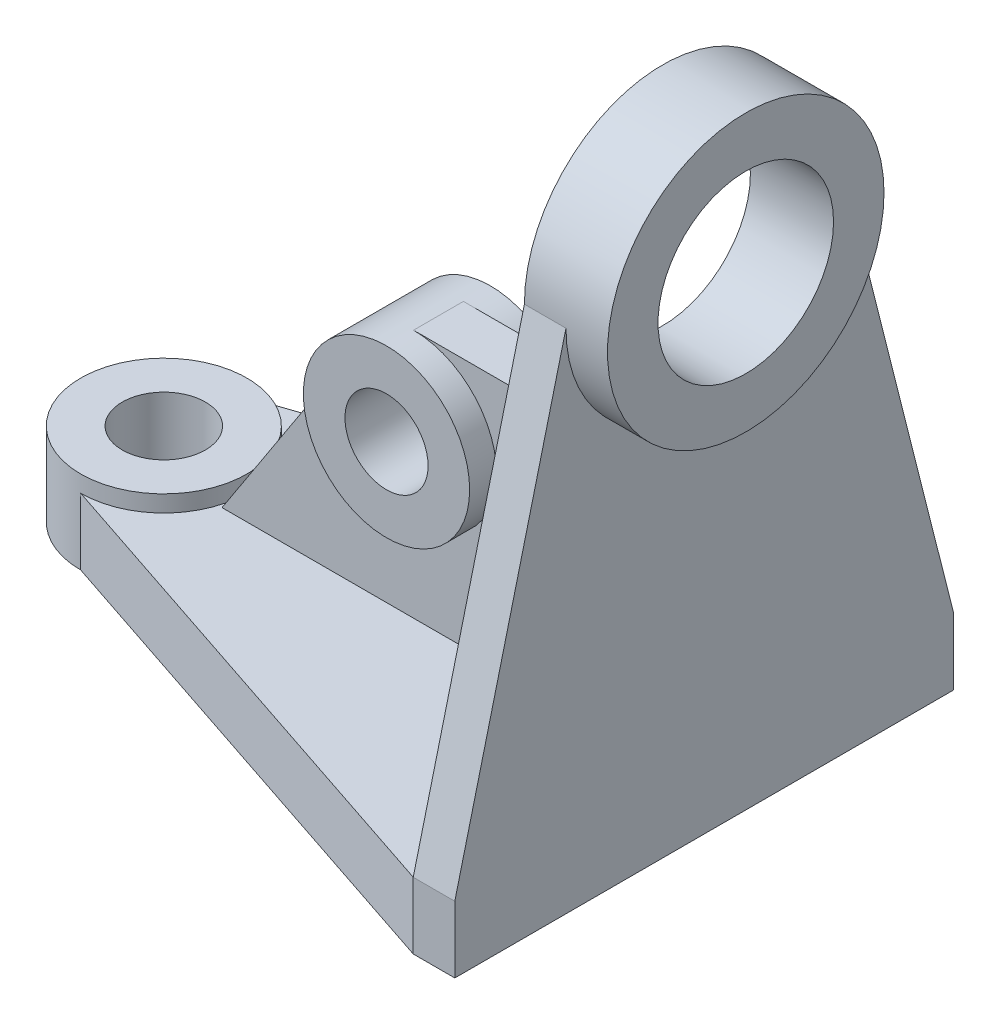
ISO-10303-21;
HEADER;
FILE_DESCRIPTION(('STEP AP214'),'2;1');
FILE_NAME('part.step','',(''),(''),'','','');
FILE_SCHEMA(('AUTOMOTIVE_DESIGN { 1 0 10303 214 1 1 1 1 }'));
ENDSEC;
DATA;
#1=APPLICATION_CONTEXT('core data for automotive mechanical design processes');
#2=APPLICATION_PROTOCOL_DEFINITION('international standard','automotive_design',2000,#1);
#3=PRODUCT_CONTEXT('',#1,'mechanical');
#4=PRODUCT('Part','Part','',(#3));
#5=PRODUCT_RELATED_PRODUCT_CATEGORY('part','',(#4));
#6=PRODUCT_DEFINITION_FORMATION('','',#4);
#7=PRODUCT_DEFINITION_CONTEXT('part definition',#1,'design');
#8=PRODUCT_DEFINITION('design','',#6,#7);
#9=PRODUCT_DEFINITION_SHAPE('','',#8);
#10=(LENGTH_UNIT() NAMED_UNIT(*) SI_UNIT(.MILLI.,.METRE.));
#11=(NAMED_UNIT(*) PLANE_ANGLE_UNIT() SI_UNIT($,.RADIAN.));
#12=(NAMED_UNIT(*) SI_UNIT($,.STERADIAN.) SOLID_ANGLE_UNIT());
#13=UNCERTAINTY_MEASURE_WITH_UNIT(LENGTH_MEASURE(1.E-05),#10,'distance_accuracy_value','');
#14=(GEOMETRIC_REPRESENTATION_CONTEXT(3) GLOBAL_UNCERTAINTY_ASSIGNED_CONTEXT((#13)) GLOBAL_UNIT_ASSIGNED_CONTEXT((#10,
#11,#12)) REPRESENTATION_CONTEXT('',''));
#15=CARTESIAN_POINT('',(0.,0.,0.));
#16=DIRECTION('',(0.,0.,1.));
#17=DIRECTION('',(1.,0.,0.));
#18=AXIS2_PLACEMENT_3D('',#15,#16,#17);
#19=CARTESIAN_POINT('',(0.,16.,0.));
#20=DIRECTION('',(0.,-1.,0.));
#21=DIRECTION('',(0.,0.,-1.));
#22=AXIS2_PLACEMENT_3D('',#19,#20,#21);
#23=PLANE('',#22);
#24=DIRECTION('',(1.,0.,0.));
#25=VECTOR('',#24,1.);
#26=CARTESIAN_POINT('',(120.,16.,6.));
#27=LINE('',#26,#25);
#28=CARTESIAN_POINT('',(20.,16.,6.));
#29=VERTEX_POINT('',#28);
#30=CARTESIAN_POINT('',(120.,16.,6.));
#31=VERTEX_POINT('',#30);
#32=EDGE_CURVE('E287',#29,#31,#27,.T.);
#33=ORIENTED_EDGE('',*,*,#32,.F.);
#34=DIRECTION('',(0.,0.,-1.));
#35=VECTOR('',#34,1.);
#36=CARTESIAN_POINT('',(20.,16.,6.));
#37=LINE('',#36,#35);
#38=CARTESIAN_POINT('',(20.,16.,0.));
#39=VERTEX_POINT('',#38);
#40=EDGE_CURVE('E170',#29,#39,#37,.T.);
#41=ORIENTED_EDGE('',*,*,#40,.T.);
#42=CARTESIAN_POINT('',(0.,16.,0.));
#43=DIRECTION('',(0.,-1.,0.));
#44=DIRECTION('',(0.,0.,-1.));
#45=AXIS2_PLACEMENT_3D('',#42,#43,#44);
#46=CIRCLE('',#45,20.);
#47=CARTESIAN_POINT('',(0.,16.,20.));
#48=VERTEX_POINT('',#47);
#49=EDGE_CURVE('E64',#39,#48,#46,.T.);
#50=ORIENTED_EDGE('',*,*,#49,.T.);
#51=DIRECTION('',(0.948683298050514,0.,0.316227766016838));
#52=VECTOR('',#51,1.);
#53=CARTESIAN_POINT('',(0.,16.,20.));
#54=LINE('',#53,#52);
#55=CARTESIAN_POINT('',(120.,16.,60.));
#56=VERTEX_POINT('',#55);
#57=EDGE_CURVE('E217',#48,#56,#54,.T.);
#58=ORIENTED_EDGE('',*,*,#57,.T.);
#59=DIRECTION('',(0.,0.,-1.));
#60=VECTOR('',#59,1.);
#61=CARTESIAN_POINT('',(120.,16.,0.));
#62=LINE('',#61,#60);
#63=EDGE_CURVE('E189',#56,#31,#62,.T.);
#64=ORIENTED_EDGE('',*,*,#63,.T.);
#65=EDGE_LOOP('',(#33,#41,#50,#58,#64));
#66=FACE_BOUND('',#65,.T.);
#67=ADVANCED_FACE('F41',(#66),#23,.F.);
#68=CARTESIAN_POINT('',(20.,16.,-6.));
#69=VERTEX_POINT('',#68);
#70=EDGE_CURVE('E163',#39,#69,#37,.T.);
#71=ORIENTED_EDGE('',*,*,#70,.T.);
#72=DIRECTION('',(1.,0.,0.));
#73=VECTOR('',#72,1.);
#74=CARTESIAN_POINT('',(120.,16.,-6.));
#75=LINE('',#74,#73);
#76=CARTESIAN_POINT('',(120.,16.,-6.));
#77=VERTEX_POINT('',#76);
#78=EDGE_CURVE('E294',#69,#77,#75,.T.);
#79=ORIENTED_EDGE('',*,*,#78,.T.);
#80=CARTESIAN_POINT('',(120.,16.,-60.));
#81=VERTEX_POINT('',#80);
#82=EDGE_CURVE('E187',#77,#81,#62,.T.);
#83=ORIENTED_EDGE('',*,*,#82,.T.);
#84=DIRECTION('',(-0.948683298050514,0.,0.316227766016838));
#85=VECTOR('',#84,1.);
#86=CARTESIAN_POINT('',(0.,16.,-20.));
#87=LINE('',#86,#85);
#88=CARTESIAN_POINT('',(0.,16.,-20.));
#89=VERTEX_POINT('',#88);
#90=EDGE_CURVE('E209',#81,#89,#87,.T.);
#91=ORIENTED_EDGE('',*,*,#90,.T.);
#92=EDGE_CURVE('E214',#89,#39,#46,.T.);
#93=ORIENTED_EDGE('',*,*,#92,.T.);
#94=EDGE_LOOP('',(#71,#79,#83,#91,#93));
#95=FACE_BOUND('',#94,.T.);
#96=ADVANCED_FACE('F301',(#95),#23,.F.);
#97=CARTESIAN_POINT('',(120.,0.,0.));
#98=DIRECTION('',(1.,0.,0.));
#99=DIRECTION('',(0.,0.,-1.));
#100=AXIS2_PLACEMENT_3D('',#97,#98,#99);
#101=PLANE('',#100);
#102=CARTESIAN_POINT('',(120.,122.,0.));
#103=DIRECTION('',(1.,0.,0.));
#104=DIRECTION('',(0.,0.,-1.));
#105=AXIS2_PLACEMENT_3D('',#102,#103,#104);
#106=CIRCLE('',#105,21.1123106954547);
#107=CARTESIAN_POINT('',(120.,122.,-21.1123106954547));
#108=VERTEX_POINT('',#107);
#109=EDGE_CURVE('E171',#108,#108,#106,.T.);
#110=ORIENTED_EDGE('',*,*,#109,.T.);
#111=EDGE_LOOP('',(#110));
#112=FACE_BOUND('',#111,.T.);
#113=DIRECTION('',(0.,1.,0.));
#114=VECTOR('',#113,1.);
#115=CARTESIAN_POINT('',(120.,76.,6.));
#116=LINE('',#115,#114);
#117=CARTESIAN_POINT('',(120.,76.,6.));
#118=VERTEX_POINT('',#117);
#119=EDGE_CURVE('E161',#31,#118,#116,.T.);
#120=ORIENTED_EDGE('',*,*,#119,.F.);
#121=ORIENTED_EDGE('',*,*,#63,.F.);
#122=DIRECTION('',(0.,0.969620280754232,-0.244615026419239));
#123=VECTOR('',#122,1.);
#124=CARTESIAN_POINT('',(120.,15.1884056140009,60.2047483804881));
#125=LINE('',#124,#123);
#126=CARTESIAN_POINT('',(120.,122.,33.2584050528832));
#127=VERTEX_POINT('',#126);
#128=EDGE_CURVE('E182',#56,#127,#125,.T.);
#129=ORIENTED_EDGE('',*,*,#128,.T.);
#130=CARTESIAN_POINT('',(120.,122.,0.));
#131=DIRECTION('',(1.,0.,0.));
#132=DIRECTION('',(0.,0.,-1.));
#133=AXIS2_PLACEMENT_3D('',#130,#131,#132);
#134=CIRCLE('',#133,33.2584050528832);
#135=CARTESIAN_POINT('',(120.,122.,-33.2584050528833));
#136=VERTEX_POINT('',#135);
#137=EDGE_CURVE('E174',#136,#127,#134,.T.);
#138=ORIENTED_EDGE('',*,*,#137,.F.);
#139=DIRECTION('',(0.,0.969620280754232,0.244615026419239));
#140=VECTOR('',#139,1.);
#141=CARTESIAN_POINT('',(120.,15.1884056140009,-60.2047483804881));
#142=LINE('',#141,#140);
#143=EDGE_CURVE('E192',#81,#136,#142,.T.);
#144=ORIENTED_EDGE('',*,*,#143,.F.);
#145=ORIENTED_EDGE('',*,*,#82,.F.);
#146=DIRECTION('',(0.,1.,0.));
#147=VECTOR('',#146,1.);
#148=CARTESIAN_POINT('',(120.,76.,-6.));
#149=LINE('',#148,#147);
#150=CARTESIAN_POINT('',(120.,76.,-6.));
#151=VERTEX_POINT('',#150);
#152=EDGE_CURVE('E154',#77,#151,#149,.T.);
#153=ORIENTED_EDGE('',*,*,#152,.T.);
#154=DIRECTION('',(0.,0.,-1.));
#155=VECTOR('',#154,1.);
#156=CARTESIAN_POINT('',(120.,76.,6.));
#157=LINE('',#156,#155);
#158=EDGE_CURVE('E148',#118,#151,#157,.T.);
#159=ORIENTED_EDGE('',*,*,#158,.F.);
#160=EDGE_LOOP('',(#120,#121,#129,#138,#144,#145,#153,#159));
#161=FACE_BOUND('',#160,.T.);
#162=ADVANCED_FACE('F281',(#112,#161),#101,.F.);
#163=CARTESIAN_POINT('',(0.,20.,0.));
#164=DIRECTION('',(0.,-1.,0.));
#165=DIRECTION('',(0.,0.,-1.));
#166=AXIS2_PLACEMENT_3D('',#163,#164,#165);
#167=CYLINDRICAL_SURFACE('',#166,20.);
#168=CARTESIAN_POINT('',(0.,20.,0.));
#169=DIRECTION('',(0.,1.,0.));
#170=DIRECTION('',(0.,0.,1.));
#171=AXIS2_PLACEMENT_3D('',#168,#169,#170);
#172=CIRCLE('',#171,20.);
#173=CARTESIAN_POINT('',(0.,20.,20.));
#174=VERTEX_POINT('',#173);
#175=EDGE_CURVE('E47',#174,#174,#172,.T.);
#176=ORIENTED_EDGE('',*,*,#175,.F.);
#177=EDGE_LOOP('',(#176));
#178=FACE_BOUND('',#177,.T.);
#179=DIRECTION('',(0.,-1.,0.));
#180=VECTOR('',#179,1.);
#181=CARTESIAN_POINT('',(0.,16.,-20.));
#182=LINE('',#181,#180);
#183=CARTESIAN_POINT('',(0.,0.,-20.));
#184=VERTEX_POINT('',#183);
#185=EDGE_CURVE('E239',#89,#184,#182,.T.);
#186=ORIENTED_EDGE('',*,*,#185,.T.);
#187=CARTESIAN_POINT('',(0.,0.,0.));
#188=DIRECTION('',(0.,1.,0.));
#189=DIRECTION('',(0.,0.,1.));
#190=AXIS2_PLACEMENT_3D('',#187,#188,#189);
#191=CIRCLE('',#190,20.);
#192=CARTESIAN_POINT('',(0.,0.,20.));
#193=VERTEX_POINT('',#192);
#194=EDGE_CURVE('E254',#184,#193,#191,.T.);
#195=ORIENTED_EDGE('',*,*,#194,.T.);
#196=DIRECTION('',(0.,-1.,0.));
#197=VECTOR('',#196,1.);
#198=CARTESIAN_POINT('',(0.,16.,20.));
#199=LINE('',#198,#197);
#200=EDGE_CURVE('E240',#48,#193,#199,.T.);
#201=ORIENTED_EDGE('',*,*,#200,.F.);
#202=ORIENTED_EDGE('',*,*,#49,.F.);
#203=ORIENTED_EDGE('',*,*,#92,.F.);
#204=EDGE_LOOP('',(#186,#195,#201,#202,#203));
#205=FACE_BOUND('',#204,.T.);
#206=ADVANCED_FACE('F43',(#178,#205),#167,.T.);
#207=CARTESIAN_POINT('',(0.,20.,0.));
#208=DIRECTION('',(0.,1.,0.));
#209=DIRECTION('',(0.,0.,1.));
#210=AXIS2_PLACEMENT_3D('',#207,#208,#209);
#211=PLANE('',#210);
#212=ORIENTED_EDGE('',*,*,#175,.T.);
#213=EDGE_LOOP('',(#212));
#214=FACE_BOUND('',#213,.T.);
#215=CARTESIAN_POINT('',(0.,20.,0.));
#216=DIRECTION('',(0.,1.,0.));
#217=DIRECTION('',(0.,0.,1.));
#218=AXIS2_PLACEMENT_3D('',#215,#216,#217);
#219=CIRCLE('',#218,10.);
#220=CARTESIAN_POINT('',(0.,20.,10.));
#221=VERTEX_POINT('',#220);
#222=EDGE_CURVE('E249',#221,#221,#219,.T.);
#223=ORIENTED_EDGE('',*,*,#222,.F.);
#224=EDGE_LOOP('',(#223));
#225=FACE_BOUND('',#224,.T.);
#226=ADVANCED_FACE('F361',(#214,#225),#211,.T.);
#227=CARTESIAN_POINT('',(0.,0.,0.));
#228=DIRECTION('',(0.,1.,0.));
#229=DIRECTION('',(0.,0.,1.));
#230=AXIS2_PLACEMENT_3D('',#227,#228,#229);
#231=PLANE('',#230);
#232=ORIENTED_EDGE('',*,*,#194,.F.);
#233=DIRECTION('',(-0.948683298050514,0.,0.316227766016838));
#234=VECTOR('',#233,1.);
#235=CARTESIAN_POINT('',(0.,0.,-20.));
#236=LINE('',#235,#234);
#237=CARTESIAN_POINT('',(120.,0.,-60.));
#238=VERTEX_POINT('',#237);
#239=EDGE_CURVE('E228',#238,#184,#236,.T.);
#240=ORIENTED_EDGE('',*,*,#239,.F.);
#241=DIRECTION('',(-1.,0.,0.));
#242=VECTOR('',#241,1.);
#243=CARTESIAN_POINT('',(120.,0.,-60.));
#244=LINE('',#243,#242);
#245=CARTESIAN_POINT('',(130.,0.,-60.));
#246=VERTEX_POINT('',#245);
#247=EDGE_CURVE('E221',#246,#238,#244,.T.);
#248=ORIENTED_EDGE('',*,*,#247,.F.);
#249=DIRECTION('',(0.,0.,-1.));
#250=VECTOR('',#249,1.);
#251=CARTESIAN_POINT('',(130.,0.,-60.));
#252=LINE('',#251,#250);
#253=CARTESIAN_POINT('',(130.,0.,60.));
#254=VERTEX_POINT('',#253);
#255=EDGE_CURVE('E201',#254,#246,#252,.T.);
#256=ORIENTED_EDGE('',*,*,#255,.F.);
#257=DIRECTION('',(1.,0.,0.));
#258=VECTOR('',#257,1.);
#259=CARTESIAN_POINT('',(130.,0.,60.));
#260=LINE('',#259,#258);
#261=CARTESIAN_POINT('',(120.,0.,60.));
#262=VERTEX_POINT('',#261);
#263=EDGE_CURVE('E208',#262,#254,#260,.T.);
#264=ORIENTED_EDGE('',*,*,#263,.F.);
#265=DIRECTION('',(0.948683298050514,0.,0.316227766016838));
#266=VECTOR('',#265,1.);
#267=CARTESIAN_POINT('',(0.,0.,20.));
#268=LINE('',#267,#266);
#269=EDGE_CURVE('E230',#193,#262,#268,.T.);
#270=ORIENTED_EDGE('',*,*,#269,.F.);
#271=EDGE_LOOP('',(#232,#240,#248,#256,#264,#270));
#272=FACE_BOUND('',#271,.T.);
#273=CARTESIAN_POINT('',(0.,0.,0.));
#274=DIRECTION('',(0.,1.,0.));
#275=DIRECTION('',(0.,0.,1.));
#276=AXIS2_PLACEMENT_3D('',#273,#274,#275);
#277=CIRCLE('',#276,10.);
#278=CARTESIAN_POINT('',(0.,0.,10.));
#279=VERTEX_POINT('',#278);
#280=EDGE_CURVE('E248',#279,#279,#277,.T.);
#281=ORIENTED_EDGE('',*,*,#280,.T.);
#282=EDGE_LOOP('',(#281));
#283=FACE_BOUND('',#282,.T.);
#284=ADVANCED_FACE('F269',(#272,#283),#231,.F.);
#285=CARTESIAN_POINT('',(0.,20.,0.));
#286=DIRECTION('',(0.,-1.,0.));
#287=DIRECTION('',(0.,0.,-1.));
#288=AXIS2_PLACEMENT_3D('',#285,#286,#287);
#289=CYLINDRICAL_SURFACE('',#288,10.);
#290=ORIENTED_EDGE('',*,*,#222,.T.);
#291=EDGE_LOOP('',(#290));
#292=FACE_BOUND('',#291,.T.);
#293=ORIENTED_EDGE('',*,*,#280,.F.);
#294=EDGE_LOOP('',(#293));
#295=FACE_BOUND('',#294,.T.);
#296=ADVANCED_FACE('F360',(#292,#295),#289,.F.);
#297=CARTESIAN_POINT('',(130.,16.,-60.));
#298=DIRECTION('',(-1.,0.,0.));
#299=DIRECTION('',(0.,0.,1.));
#300=AXIS2_PLACEMENT_3D('',#297,#298,#299);
#301=PLANE('',#300);
#302=ORIENTED_EDGE('',*,*,#255,.T.);
#303=DIRECTION('',(0.,-1.,0.));
#304=VECTOR('',#303,1.);
#305=CARTESIAN_POINT('',(130.,16.,-60.));
#306=LINE('',#305,#304);
#307=CARTESIAN_POINT('',(130.,16.,-60.));
#308=VERTEX_POINT('',#307);
#309=EDGE_CURVE('E246',#308,#246,#306,.T.);
#310=ORIENTED_EDGE('',*,*,#309,.F.);
#311=DIRECTION('',(0.,0.969620280754232,0.244615026419239));
#312=VECTOR('',#311,1.);
#313=CARTESIAN_POINT('',(130.,15.1884056140009,-60.2047483804881));
#314=LINE('',#313,#312);
#315=CARTESIAN_POINT('',(130.,122.,-33.2584050528832));
#316=VERTEX_POINT('',#315);
#317=EDGE_CURVE('E190',#308,#316,#314,.T.);
#318=ORIENTED_EDGE('',*,*,#317,.T.);
#319=CARTESIAN_POINT('',(130.,122.,0.));
#320=DIRECTION('',(1.,0.,0.));
#321=DIRECTION('',(0.,0.,-1.));
#322=AXIS2_PLACEMENT_3D('',#319,#320,#321);
#323=CIRCLE('',#322,33.2584050528832);
#324=CARTESIAN_POINT('',(130.,122.,33.2584050528832));
#325=VERTEX_POINT('',#324);
#326=EDGE_CURVE('E181',#325,#316,#323,.T.);
#327=ORIENTED_EDGE('',*,*,#326,.F.);
#328=DIRECTION('',(0.,0.969620280754232,-0.244615026419239));
#329=VECTOR('',#328,1.);
#330=CARTESIAN_POINT('',(130.,15.1884056140009,60.2047483804881));
#331=LINE('',#330,#329);
#332=CARTESIAN_POINT('',(130.,16.,60.));
#333=VERTEX_POINT('',#332);
#334=EDGE_CURVE('E197',#333,#325,#331,.T.);
#335=ORIENTED_EDGE('',*,*,#334,.F.);
#336=DIRECTION('',(0.,-1.,0.));
#337=VECTOR('',#336,1.);
#338=CARTESIAN_POINT('',(130.,16.,60.));
#339=LINE('',#338,#337);
#340=EDGE_CURVE('E222',#333,#254,#339,.T.);
#341=ORIENTED_EDGE('',*,*,#340,.T.);
#342=EDGE_LOOP('',(#302,#310,#318,#327,#335,#341));
#343=FACE_BOUND('',#342,.T.);
#344=ADVANCED_FACE('F273',(#343),#301,.F.);
#345=CARTESIAN_POINT('',(120.,16.,-60.));
#346=DIRECTION('',(0.,0.,1.));
#347=DIRECTION('',(1.,0.,0.));
#348=AXIS2_PLACEMENT_3D('',#345,#346,#347);
#349=PLANE('',#348);
#350=ORIENTED_EDGE('',*,*,#247,.T.);
#351=DIRECTION('',(0.,-1.,0.));
#352=VECTOR('',#351,1.);
#353=CARTESIAN_POINT('',(120.,16.,-60.));
#354=LINE('',#353,#352);
#355=EDGE_CURVE('E243',#81,#238,#354,.T.);
#356=ORIENTED_EDGE('',*,*,#355,.F.);
#357=DIRECTION('',(-1.,0.,0.));
#358=VECTOR('',#357,1.);
#359=CARTESIAN_POINT('',(120.,16.,-60.));
#360=LINE('',#359,#358);
#361=EDGE_CURVE('E207',#308,#81,#360,.T.);
#362=ORIENTED_EDGE('',*,*,#361,.F.);
#363=ORIENTED_EDGE('',*,*,#309,.T.);
#364=EDGE_LOOP('',(#350,#356,#362,#363));
#365=FACE_BOUND('',#364,.T.);
#366=ADVANCED_FACE('F354',(#365),#349,.F.);
#367=CARTESIAN_POINT('',(0.,16.,-20.));
#368=DIRECTION('',(0.316227766016838,0.,0.948683298050514));
#369=DIRECTION('',(0.948683298050514,0.,-0.316227766016838));
#370=AXIS2_PLACEMENT_3D('',#367,#368,#369);
#371=PLANE('',#370);
#372=ORIENTED_EDGE('',*,*,#239,.T.);
#373=ORIENTED_EDGE('',*,*,#185,.F.);
#374=ORIENTED_EDGE('',*,*,#90,.F.);
#375=ORIENTED_EDGE('',*,*,#355,.T.);
#376=EDGE_LOOP('',(#372,#373,#374,#375));
#377=FACE_BOUND('',#376,.T.);
#378=ADVANCED_FACE('F346',(#377),#371,.F.);
#379=CARTESIAN_POINT('',(0.,16.,20.));
#380=DIRECTION('',(0.316227766016838,0.,-0.948683298050514));
#381=DIRECTION('',(-0.948683298050514,0.,-0.316227766016838));
#382=AXIS2_PLACEMENT_3D('',#379,#380,#381);
#383=PLANE('',#382);
#384=ORIENTED_EDGE('',*,*,#269,.T.);
#385=DIRECTION('',(0.,-1.,0.));
#386=VECTOR('',#385,1.);
#387=CARTESIAN_POINT('',(120.,16.,60.));
#388=LINE('',#387,#386);
#389=EDGE_CURVE('E234',#56,#262,#388,.T.);
#390=ORIENTED_EDGE('',*,*,#389,.F.);
#391=ORIENTED_EDGE('',*,*,#57,.F.);
#392=ORIENTED_EDGE('',*,*,#200,.T.);
#393=EDGE_LOOP('',(#384,#390,#391,#392));
#394=FACE_BOUND('',#393,.T.);
#395=ADVANCED_FACE('F261',(#394),#383,.F.);
#396=CARTESIAN_POINT('',(130.,16.,60.));
#397=DIRECTION('',(0.,0.,-1.));
#398=DIRECTION('',(-1.,0.,0.));
#399=AXIS2_PLACEMENT_3D('',#396,#397,#398);
#400=PLANE('',#399);
#401=ORIENTED_EDGE('',*,*,#263,.T.);
#402=ORIENTED_EDGE('',*,*,#340,.F.);
#403=DIRECTION('',(1.,0.,0.));
#404=VECTOR('',#403,1.);
#405=CARTESIAN_POINT('',(130.,16.,60.));
#406=LINE('',#405,#404);
#407=EDGE_CURVE('E219',#56,#333,#406,.T.);
#408=ORIENTED_EDGE('',*,*,#407,.F.);
#409=ORIENTED_EDGE('',*,*,#389,.T.);
#410=EDGE_LOOP('',(#401,#402,#408,#409));
#411=FACE_BOUND('',#410,.T.);
#412=ADVANCED_FACE('F272',(#411),#400,.F.);
#413=CARTESIAN_POINT('',(120.,15.1884056140009,-60.2047483804881));
#414=DIRECTION('',(0.,0.244615026419239,-0.969620280754232));
#415=DIRECTION('',(0.,0.969620280754232,0.244615026419239));
#416=AXIS2_PLACEMENT_3D('',#413,#414,#415);
#417=PLANE('',#416);
#418=ORIENTED_EDGE('',*,*,#317,.F.);
#419=ORIENTED_EDGE('',*,*,#361,.T.);
#420=ORIENTED_EDGE('',*,*,#143,.T.);
#421=DIRECTION('',(1.,0.,0.));
#422=VECTOR('',#421,1.);
#423=CARTESIAN_POINT('',(120.,122.,-33.2584050528833));
#424=LINE('',#423,#422);
#425=EDGE_CURVE('E202',#136,#316,#424,.T.);
#426=ORIENTED_EDGE('',*,*,#425,.T.);
#427=EDGE_LOOP('',(#418,#419,#420,#426));
#428=FACE_BOUND('',#427,.T.);
#429=ADVANCED_FACE('F347',(#428),#417,.T.);
#430=CARTESIAN_POINT('',(120.,15.1884056140009,60.2047483804881));
#431=DIRECTION('',(0.,-0.244615026419239,-0.969620280754232));
#432=DIRECTION('',(0.,0.969620280754232,-0.244615026419239));
#433=AXIS2_PLACEMENT_3D('',#430,#431,#432);
#434=PLANE('',#433);
#435=ORIENTED_EDGE('',*,*,#334,.T.);
#436=DIRECTION('',(1.,0.,0.));
#437=VECTOR('',#436,1.);
#438=CARTESIAN_POINT('',(120.,122.,33.2584050528833));
#439=LINE('',#438,#437);
#440=EDGE_CURVE('E191',#127,#325,#439,.T.);
#441=ORIENTED_EDGE('',*,*,#440,.F.);
#442=ORIENTED_EDGE('',*,*,#128,.F.);
#443=ORIENTED_EDGE('',*,*,#407,.T.);
#444=EDGE_LOOP('',(#435,#441,#442,#443));
#445=FACE_BOUND('',#444,.T.);
#446=ADVANCED_FACE('F276',(#445),#434,.F.);
#447=CARTESIAN_POINT('',(140.,122.,0.));
#448=DIRECTION('',(1.,0.,0.));
#449=DIRECTION('',(0.,0.,-1.));
#450=AXIS2_PLACEMENT_3D('',#447,#448,#449);
#451=PLANE('',#450);
#452=CARTESIAN_POINT('',(140.,122.,0.));
#453=DIRECTION('',(1.,0.,0.));
#454=DIRECTION('',(0.,0.,-1.));
#455=AXIS2_PLACEMENT_3D('',#452,#453,#454);
#456=CIRCLE('',#455,33.2584050528832);
#457=CARTESIAN_POINT('',(140.,122.,-33.2584050528832));
#458=VERTEX_POINT('',#457);
#459=EDGE_CURVE('E178',#458,#458,#456,.T.);
#460=ORIENTED_EDGE('',*,*,#459,.T.);
#461=EDGE_LOOP('',(#460));
#462=FACE_BOUND('',#461,.T.);
#463=CARTESIAN_POINT('',(140.,122.,0.));
#464=DIRECTION('',(1.,0.,0.));
#465=DIRECTION('',(0.,0.,-1.));
#466=AXIS2_PLACEMENT_3D('',#463,#464,#465);
#467=CIRCLE('',#466,21.1123106954547);
#468=CARTESIAN_POINT('',(140.,122.,-21.1123106954547));
#469=VERTEX_POINT('',#468);
#470=EDGE_CURVE('E175',#469,#469,#467,.T.);
#471=ORIENTED_EDGE('',*,*,#470,.F.);
#472=EDGE_LOOP('',(#471));
#473=FACE_BOUND('',#472,.T.);
#474=ADVANCED_FACE('F414',(#462,#473),#451,.T.);
#475=CARTESIAN_POINT('',(140.,122.,0.));
#476=DIRECTION('',(-1.,0.,0.));
#477=DIRECTION('',(0.,0.,1.));
#478=AXIS2_PLACEMENT_3D('',#475,#476,#477);
#479=CYLINDRICAL_SURFACE('',#478,33.2584050528832);
#480=ORIENTED_EDGE('',*,*,#425,.F.);
#481=ORIENTED_EDGE('',*,*,#137,.T.);
#482=ORIENTED_EDGE('',*,*,#440,.T.);
#483=ORIENTED_EDGE('',*,*,#326,.T.);
#484=EDGE_LOOP('',(#480,#481,#482,#483));
#485=FACE_BOUND('',#484,.T.);
#486=ORIENTED_EDGE('',*,*,#459,.F.);
#487=EDGE_LOOP('',(#486));
#488=FACE_BOUND('',#487,.T.);
#489=ADVANCED_FACE('F423',(#485,#488),#479,.T.);
#490=CARTESIAN_POINT('',(140.,122.,0.));
#491=DIRECTION('',(-1.,0.,0.));
#492=DIRECTION('',(0.,0.,1.));
#493=AXIS2_PLACEMENT_3D('',#490,#491,#492);
#494=CYLINDRICAL_SURFACE('',#493,21.1123106954547);
#495=ORIENTED_EDGE('',*,*,#470,.T.);
#496=EDGE_LOOP('',(#495));
#497=FACE_BOUND('',#496,.T.);
#498=ORIENTED_EDGE('',*,*,#109,.F.);
#499=EDGE_LOOP('',(#498));
#500=FACE_BOUND('',#499,.T.);
#501=ADVANCED_FACE('F430',(#497,#500),#494,.F.);
#502=CARTESIAN_POINT('',(66.0700000000001,56.,6.));
#503=DIRECTION('',(0.,0.,-1.));
#504=DIRECTION('',(-1.,0.,0.));
#505=AXIS2_PLACEMENT_3D('',#502,#503,#504);
#506=CYLINDRICAL_SURFACE('',#505,20.);
#507=DIRECTION('',(0.,0.,-1.));
#508=VECTOR('',#507,1.);
#509=CARTESIAN_POINT('',(66.07,76.,6.));
#510=LINE('',#509,#508);
#511=CARTESIAN_POINT('',(66.07,76.,6.));
#512=VERTEX_POINT('',#511);
#513=CARTESIAN_POINT('',(66.07,76.,-6.));
#514=VERTEX_POINT('',#513);
#515=EDGE_CURVE('E150',#512,#514,#510,.T.);
#516=ORIENTED_EDGE('',*,*,#515,.T.);
#517=CARTESIAN_POINT('',(66.07,56.,-6.));
#518=DIRECTION('',(0.,0.,-1.));
#519=DIRECTION('',(-1.,0.,0.));
#520=AXIS2_PLACEMENT_3D('',#517,#518,#519);
#521=CIRCLE('',#520,20.);
#522=CARTESIAN_POINT('',(46.07,56.,-6.));
#523=VERTEX_POINT('',#522);
#524=EDGE_CURVE('E11',#523,#514,#521,.F.);
#525=ORIENTED_EDGE('',*,*,#524,.F.);
#526=DIRECTION('',(0.,0.,-1.));
#527=VECTOR('',#526,1.);
#528=CARTESIAN_POINT('',(46.07,56.,6.));
#529=LINE('',#528,#527);
#530=CARTESIAN_POINT('',(46.07,56.,6.));
#531=VERTEX_POINT('',#530);
#532=EDGE_CURVE('E169',#531,#523,#529,.T.);
#533=ORIENTED_EDGE('',*,*,#532,.F.);
#534=CARTESIAN_POINT('',(66.07,56.,6.));
#535=DIRECTION('',(0.,0.,-1.));
#536=DIRECTION('',(-1.,0.,0.));
#537=AXIS2_PLACEMENT_3D('',#534,#535,#536);
#538=CIRCLE('',#537,20.);
#539=EDGE_CURVE('E160',#531,#512,#538,.F.);
#540=ORIENTED_EDGE('',*,*,#539,.T.);
#541=EDGE_LOOP('',(#516,#525,#533,#540));
#542=FACE_BOUND('',#541,.T.);
#543=CARTESIAN_POINT('',(66.07,56.,-12.5));
#544=DIRECTION('',(0.,0.,1.));
#545=DIRECTION('',(1.,0.,0.));
#546=AXIS2_PLACEMENT_3D('',#543,#544,#545);
#547=CIRCLE('',#546,20.);
#548=CARTESIAN_POINT('',(86.07,56.,-12.5));
#549=VERTEX_POINT('',#548);
#550=EDGE_CURVE('E307',#549,#549,#547,.T.);
#551=ORIENTED_EDGE('',*,*,#550,.T.);
#552=EDGE_LOOP('',(#551));
#553=FACE_BOUND('',#552,.T.);
#554=CARTESIAN_POINT('',(66.07,56.,12.5));
#555=DIRECTION('',(0.,0.,1.));
#556=DIRECTION('',(1.,0.,0.));
#557=AXIS2_PLACEMENT_3D('',#554,#555,#556);
#558=CIRCLE('',#557,20.);
#559=CARTESIAN_POINT('',(86.07,56.,12.5));
#560=VERTEX_POINT('',#559);
#561=EDGE_CURVE('E310',#560,#560,#558,.T.);
#562=ORIENTED_EDGE('',*,*,#561,.F.);
#563=EDGE_LOOP('',(#562));
#564=FACE_BOUND('',#563,.T.);
#565=ADVANCED_FACE('F153',(#542,#553,#564),#506,.T.);
#566=CARTESIAN_POINT('',(20.,16.,6.));
#567=DIRECTION('',(0.837773058863527,-0.546018591114304,0.));
#568=DIRECTION('',(0.546018591114304,0.837773058863527,0.));
#569=AXIS2_PLACEMENT_3D('',#566,#567,#568);
#570=PLANE('',#569);
#571=DIRECTION('',(-0.546018591114304,-0.837773058863527,0.));
#572=VECTOR('',#571,1.);
#573=CARTESIAN_POINT('',(20.,16.,-6.));
#574=LINE('',#573,#572);
#575=EDGE_CURVE('E136',#523,#69,#574,.T.);
#576=ORIENTED_EDGE('',*,*,#575,.T.);
#577=ORIENTED_EDGE('',*,*,#70,.F.);
#578=ORIENTED_EDGE('',*,*,#40,.F.);
#579=DIRECTION('',(-0.546018591114304,-0.837773058863527,0.));
#580=VECTOR('',#579,1.);
#581=CARTESIAN_POINT('',(20.,16.,6.));
#582=LINE('',#581,#580);
#583=EDGE_CURVE('E155',#531,#29,#582,.T.);
#584=ORIENTED_EDGE('',*,*,#583,.F.);
#585=ORIENTED_EDGE('',*,*,#532,.T.);
#586=EDGE_LOOP('',(#576,#577,#578,#584,#585));
#587=FACE_BOUND('',#586,.T.);
#588=ADVANCED_FACE('F302',(#587),#570,.F.);
#589=CARTESIAN_POINT('',(66.07,76.,6.));
#590=DIRECTION('',(0.,-1.,0.));
#591=DIRECTION('',(0.,0.,-1.));
#592=AXIS2_PLACEMENT_3D('',#589,#590,#591);
#593=PLANE('',#592);
#594=DIRECTION('',(-1.,0.,0.));
#595=VECTOR('',#594,1.);
#596=CARTESIAN_POINT('',(66.07,76.,-6.));
#597=LINE('',#596,#595);
#598=EDGE_CURVE('E54',#151,#514,#597,.T.);
#599=ORIENTED_EDGE('',*,*,#598,.T.);
#600=ORIENTED_EDGE('',*,*,#515,.F.);
#601=DIRECTION('',(-1.,0.,0.));
#602=VECTOR('',#601,1.);
#603=CARTESIAN_POINT('',(66.07,76.,6.));
#604=LINE('',#603,#602);
#605=EDGE_CURVE('E156',#118,#512,#604,.T.);
#606=ORIENTED_EDGE('',*,*,#605,.F.);
#607=ORIENTED_EDGE('',*,*,#158,.T.);
#608=EDGE_LOOP('',(#599,#600,#606,#607));
#609=FACE_BOUND('',#608,.T.);
#610=ADVANCED_FACE('F143',(#609),#593,.F.);
#611=CARTESIAN_POINT('',(66.0700000000001,56.,6.));
#612=DIRECTION('',(0.,0.,-1.));
#613=DIRECTION('',(-1.,0.,0.));
#614=AXIS2_PLACEMENT_3D('',#611,#612,#613);
#615=PLANE('',#614);
#616=ORIENTED_EDGE('',*,*,#539,.F.);
#617=ORIENTED_EDGE('',*,*,#583,.T.);
#618=ORIENTED_EDGE('',*,*,#32,.T.);
#619=ORIENTED_EDGE('',*,*,#119,.T.);
#620=ORIENTED_EDGE('',*,*,#605,.T.);
#621=EDGE_LOOP('',(#616,#617,#618,#619,#620));
#622=FACE_BOUND('',#621,.T.);
#623=ADVANCED_FACE('F306',(#622),#615,.F.);
#624=CARTESIAN_POINT('',(66.0700000000001,56.,-6.));
#625=DIRECTION('',(0.,0.,-1.));
#626=DIRECTION('',(-1.,0.,0.));
#627=AXIS2_PLACEMENT_3D('',#624,#625,#626);
#628=PLANE('',#627);
#629=ORIENTED_EDGE('',*,*,#575,.F.);
#630=ORIENTED_EDGE('',*,*,#524,.T.);
#631=ORIENTED_EDGE('',*,*,#598,.F.);
#632=ORIENTED_EDGE('',*,*,#152,.F.);
#633=ORIENTED_EDGE('',*,*,#78,.F.);
#634=EDGE_LOOP('',(#629,#630,#631,#632,#633));
#635=FACE_BOUND('',#634,.T.);
#636=ADVANCED_FACE('F139',(#635),#628,.T.);
#637=CARTESIAN_POINT('',(66.07,56.,-12.5));
#638=DIRECTION('',(0.,0.,1.));
#639=DIRECTION('',(1.,0.,0.));
#640=AXIS2_PLACEMENT_3D('',#637,#638,#639);
#641=PLANE('',#640);
#642=ORIENTED_EDGE('',*,*,#550,.F.);
#643=EDGE_LOOP('',(#642));
#644=FACE_BOUND('',#643,.T.);
#645=CARTESIAN_POINT('',(66.07,56.,-12.5));
#646=DIRECTION('',(0.,0.,1.));
#647=DIRECTION('',(1.,0.,0.));
#648=AXIS2_PLACEMENT_3D('',#645,#646,#647);
#649=CIRCLE('',#648,10.);
#650=CARTESIAN_POINT('',(76.07,56.,-12.5));
#651=VERTEX_POINT('',#650);
#652=EDGE_CURVE('E314',#651,#651,#649,.T.);
#653=ORIENTED_EDGE('',*,*,#652,.T.);
#654=EDGE_LOOP('',(#653));
#655=FACE_BOUND('',#654,.T.);
#656=ADVANCED_FACE('F334',(#644,#655),#641,.F.);
#657=CARTESIAN_POINT('',(66.07,56.,12.5));
#658=DIRECTION('',(0.,0.,-1.));
#659=DIRECTION('',(-1.,0.,0.));
#660=AXIS2_PLACEMENT_3D('',#657,#658,#659);
#661=CYLINDRICAL_SURFACE('',#660,10.);
#662=CARTESIAN_POINT('',(66.07,56.,12.5));
#663=DIRECTION('',(0.,0.,1.));
#664=DIRECTION('',(1.,0.,0.));
#665=AXIS2_PLACEMENT_3D('',#662,#663,#664);
#666=CIRCLE('',#665,10.);
#667=CARTESIAN_POINT('',(76.07,56.,12.5));
#668=VERTEX_POINT('',#667);
#669=EDGE_CURVE('E312',#668,#668,#666,.T.);
#670=ORIENTED_EDGE('',*,*,#669,.T.);
#671=EDGE_LOOP('',(#670));
#672=FACE_BOUND('',#671,.T.);
#673=ORIENTED_EDGE('',*,*,#652,.F.);
#674=EDGE_LOOP('',(#673));
#675=FACE_BOUND('',#674,.T.);
#676=ADVANCED_FACE('F322',(#672,#675),#661,.F.);
#677=CARTESIAN_POINT('',(66.07,56.,12.5));
#678=DIRECTION('',(0.,0.,1.));
#679=DIRECTION('',(1.,0.,0.));
#680=AXIS2_PLACEMENT_3D('',#677,#678,#679);
#681=PLANE('',#680);
#682=ORIENTED_EDGE('',*,*,#561,.T.);
#683=EDGE_LOOP('',(#682));
#684=FACE_BOUND('',#683,.T.);
#685=ORIENTED_EDGE('',*,*,#669,.F.);
#686=EDGE_LOOP('',(#685));
#687=FACE_BOUND('',#686,.T.);
#688=ADVANCED_FACE('F321',(#684,#687),#681,.T.);
#689=CLOSED_SHELL('',(#67,#96,#162,#206,#226,#284,#296,#344,#366,#378,#395,#412,#429,#446,#474,
#489,#501,#565,#588,#610,#623,#636,#656,#676,#688));
#690=MANIFOLD_SOLID_BREP('B2',#689);
#691=ADVANCED_BREP_SHAPE_REPRESENTATION('',(#18,#690),#14);
#692=SHAPE_DEFINITION_REPRESENTATION(#9,#691);
ENDSEC;
END-ISO-10303-21;
